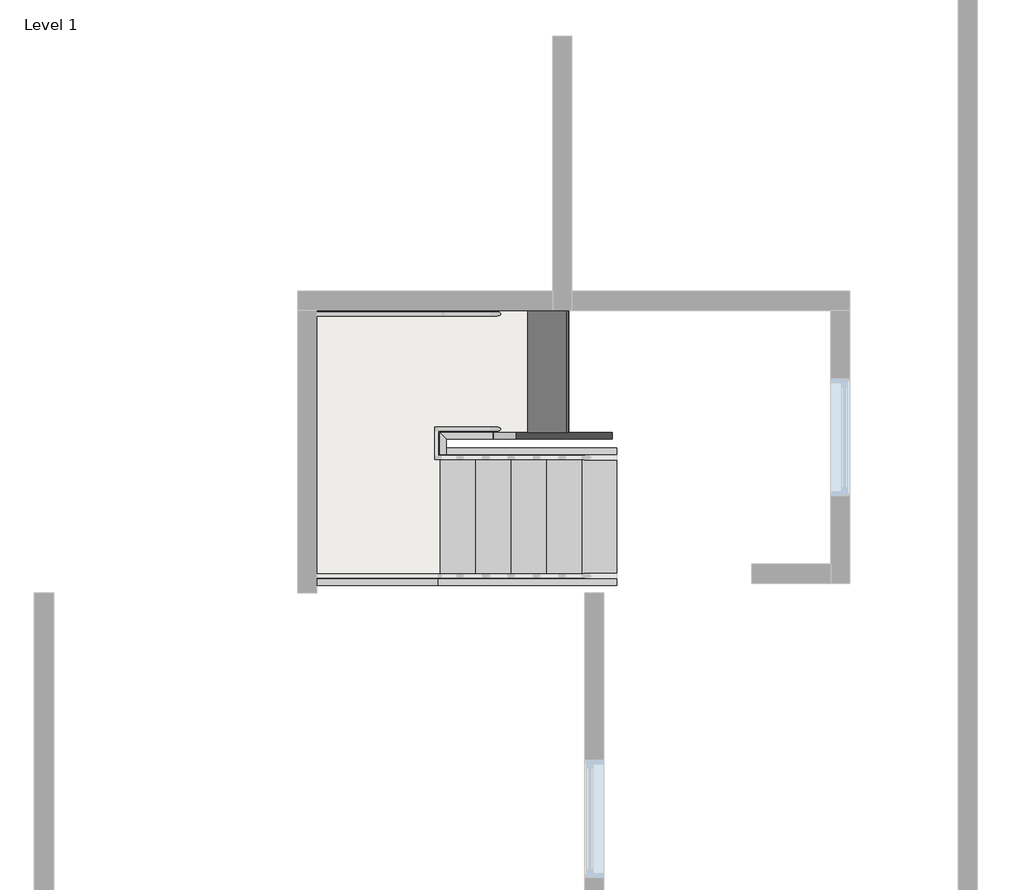
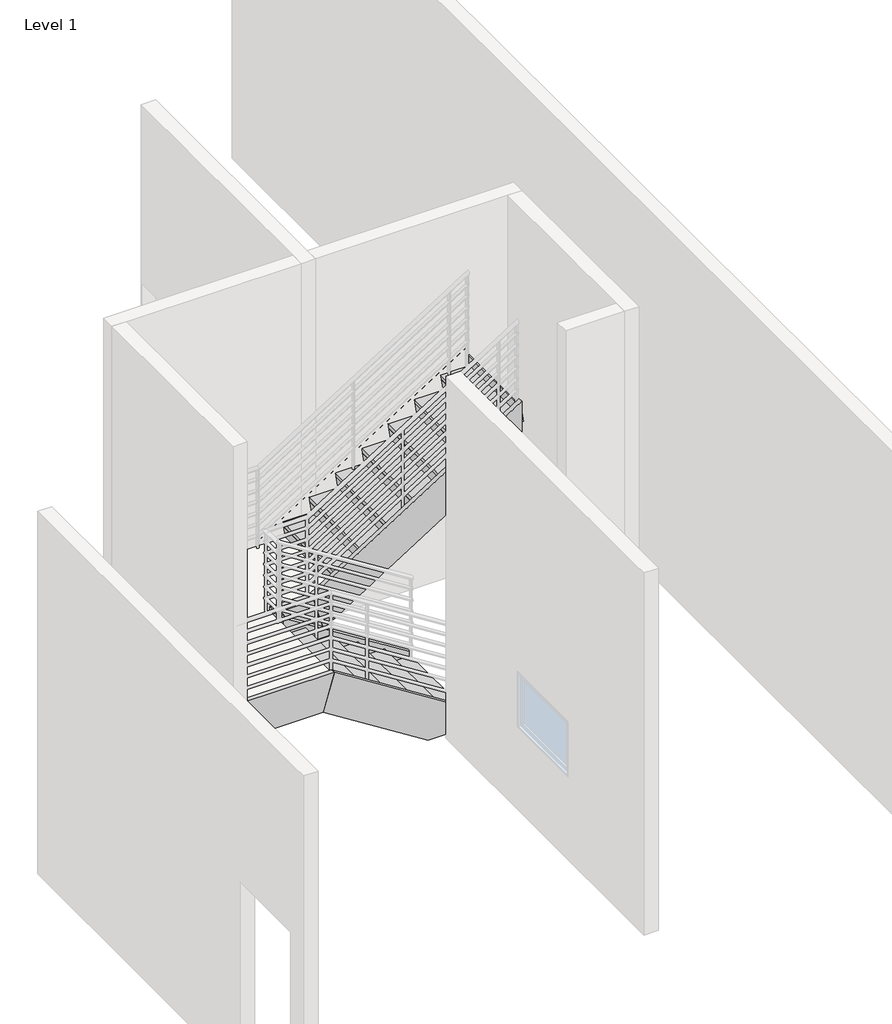
# One storey, part 4 of 4: 9 members, 2 stair flights, 1 slab.
"""IFC4 building model written with IfcOpenShell, lengths in millimetres."""

from ifc_helpers import new_model, si_unit, frame, origin, place, context, project, spatial, polyline, outline, extrude, faceted_brep, transform, mapped, element, save
from components import non_monolithic_landing_e0a5ec0f, stair_flight_50mm_tread_25mm_nosing_13mm_riser_d346f2b6, stair_flight_50mm_tread_25mm_nosing_13mm_riser_6fe2c66d

model = new_model("IFC4")

# Units and contexts
model_context = context("Model", 3, world=origin())
ifc_project = project(units=[si_unit("LENGTHUNIT", "METRE", prefix="MILLI")], contexts=[model_context])

# Site, building, storey
site = spatial("IfcSite", under=ifc_project)
building = spatial("IfcBuilding", under=site)
storey = spatial("IfcBuildingStorey", under=building, Name="Level 1", Elevation=0.0)

# Members
placement = place(None, origin())
element("IfcMember", 1, ObjectType="Stringer - 50mm Width", at=placement, inside=storey, context=model_context, shape_type="SweptSolid", body=[
    extrude(outline(polyline([(0.0, -539.0915237), (215.089535, -539.0915237), (1090.8719878, -1923.9225273), (690.8719878, -2039.7915873), (0.0, -947.3502566), (0.0, -539.0915237)])), frame((0.0, 793.0180557, 0.0), z_axis=(0.0, 1.0, 0.0), x_axis=(0.0, 0.0, 1.0)), (0.0, 0.0, 1.0), 50.0),
])
element("IfcMember", 2, ObjectType="Stringer - 50mm Width", at=placement, inside=storey, context=model_context, shape_type="SweptSolid", body=[
    extrude(outline(polyline([(0.0, -539.0915237), (215.089535, -539.0915237), (1053.034199, -1864.0915237), (579.7573231, -1864.0915237), (0.0, -947.3502566), (0.0, -539.0915237)])), frame((0.0, 1810.8567276, 0.0), z_axis=(0.0, 1.0, 0.0), x_axis=(0.0, 0.0, 1.0)), (0.0, 0.0, 1.0), 50.0),
])
element("IfcMember", 3, ObjectType="Stringer - 50mm Width", at=placement, inside=storey, context=model_context, shape_type="SweptSolid", body=[
    extrude(outline(polyline([(1090.8719878, -1497.6387118), (690.8719878, -1381.7696518), (2002.6822243, 692.5302847), (2475.9591002, 692.5302847), (1090.8719878, -1497.6387118)])), frame((0.0, 2926.2309464, 0.0), z_axis=(0.0, 1.0, 0.0), x_axis=(0.0, 0.0, 1.0)), (0.0, 0.0, 1.0), 50.0),
])
element("IfcMember", 4, ObjectType="Stringer - 50mm Width", at=placement, inside=storey, context=model_context, shape_type="SweptSolid", body=[
    extrude(outline(polyline([(1090.8719878, -1497.6387118), (690.8719878, -1381.7696518), (2002.6822243, 692.5302847), (2475.9591002, 692.5302847), (1090.8719878, -1497.6387118)])), frame((0.0, 1930.9593033, 0.0), z_axis=(0.0, 1.0, 0.0), x_axis=(0.0, 0.0, 1.0)), (0.0, 0.0, 1.0), 50.0),
])
element("IfcMember", 5, ObjectType="Stringer - 50mm Width", at=placement, inside=storey, context=model_context, shape_type="Brep", body=[
    faceted_brep([(-1497.6387118, 2926.2309464, 1090.8719878), (-1497.6387118, 2976.2309464, 1090.8719878), (-2964.117305, 2976.2309464, 1090.8719878), (-2914.117305, 2926.2309464, 1090.8719878), (-1381.7696518, 2926.2309464, 690.8719878), (-2914.117305, 2926.2309464, 690.8719878), (-1381.7696518, 2976.2309464, 690.8719878), (-2964.117305, 2976.2309464, 690.8719878)], [[[0, 1, 2, 3]], [[4, 0, 3, 5]], [[6, 4, 5, 7]], [[1, 6, 7, 2]], [[1, 0, 4, 6]], [[2, 7, 5, 3]]]),
])
element("IfcMember", 6, ObjectType="Stringer - 50mm Width", at=placement, inside=storey, context=model_context, shape_type="SweptSolid", body=[
    extrude(outline(polyline([(-2964.117305, 2976.2309464), (-2914.117305, 2926.2309464), (-2914.117305, 843.0180557), (-2964.117305, 793.0180557), (-2964.117305, 2976.2309464)])), frame((0.0, 0.0, 690.8719878), z_axis=(0.0, 0.0, 1.0), x_axis=(1.0, 0.0, 0.0)), (0.0, 0.0, 1.0), 400.0),
])
element("IfcMember", 7, ObjectType="Stringer - 50mm Width", at=placement, inside=storey, context=model_context, shape_type="Brep", body=[
    faceted_brep([(-2914.117305, 843.0180557, 1090.8719878), (-2964.117305, 793.0180557, 1090.8719878), (-1923.9225273, 793.0180557, 1090.8719878), (-1923.9225273, 843.0180557, 1090.8719878), (-2914.117305, 843.0180557, 690.8719878), (-2039.7915873, 843.0180557, 690.8719878), (-2964.117305, 793.0180557, 690.8719878), (-2039.7915873, 793.0180557, 690.8719878)], [[[0, 1, 2, 3]], [[4, 0, 3, 5]], [[6, 4, 5, 7]], [[1, 6, 7, 2]], [[1, 0, 4, 6]], [[2, 7, 5, 3]]]),
])
element("IfcMember", 8, ObjectType="Stringer - 50mm Width", at=placement, inside=storey, context=model_context, shape_type="SweptSolid", body=[
    extrude(outline(polyline([(-1864.0915237, 1810.8567276), (-1914.0915237, 1810.8567276), (-1914.0915237, 1980.9593033), (-1864.0915237, 1930.9593033), (-1864.0915237, 1810.8567276)])), frame((0.0, 0.0, 690.8719878), z_axis=(0.0, 0.0, 1.0), x_axis=(1.0, 0.0, 0.0)), (0.0, 0.0, 1.0), 400.0),
])
element("IfcMember", 9, ObjectType="Stringer - 50mm Width", at=placement, inside=storey, context=model_context, shape_type="Brep", body=[
    faceted_brep([(-1914.0915237, 1980.9593033, 1090.8719878), (-1864.0915237, 1930.9593033, 1090.8719878), (-1497.6387118, 1930.9593033, 1090.8719878), (-1497.6387118, 1980.9593033, 1090.8719878), (-1914.0915237, 1980.9593033, 690.8719878), (-1381.7696518, 1980.9593033, 690.8719878), (-1864.0915237, 1930.9593033, 690.8719878), (-1381.7696518, 1930.9593033, 690.8719878)], [[[0, 1, 2, 3]], [[4, 0, 3, 5]], [[6, 4, 5, 7]], [[1, 6, 7, 2]], [[1, 0, 4, 6]], [[2, 7, 5, 3]]]),
])

# Slab
non_monolithic_landing_shape = non_monolithic_landing_e0a5ec0f(model_context)
element("IfcSlab", 10, ObjectType="Non-Monolithic Landing", at=placement, inside=storey, context=model_context, shape_type="MappedRepresentation", body=[
    mapped(non_monolithic_landing_shape, transform((0.0, 0.0, 0.0), x_axis=(1.0, 0.0, 0.0), y_axis=(0.0, 1.0, 0.0), z_axis=(0.0, 0.0, 1.0))),
])

# Stair flights
stair_flight_50mm_tread_25mm_nosing_13mm_riser_shape = stair_flight_50mm_tread_25mm_nosing_13mm_riser_d346f2b6(model_context)
element("IfcStairFlight", 11, ObjectType="50mm Tread 25mm Nosing 13mm Riser", at=placement, inside=storey, context=model_context, shape_type="MappedRepresentation", body=[
    mapped(stair_flight_50mm_tread_25mm_nosing_13mm_riser_shape, transform((0.0, 0.0, 0.0), x_axis=(1.0, 0.0, 0.0), y_axis=(0.0, 1.0, 0.0), z_axis=(0.0, 0.0, 1.0))),
])
stair_flight_50mm_tread_25mm_nosing_13mm_riser_2_shape = stair_flight_50mm_tread_25mm_nosing_13mm_riser_6fe2c66d(model_context)
element("IfcStairFlight", 12, ObjectType="50mm Tread 25mm Nosing 13mm Riser", at=placement, inside=storey, context=model_context, shape_type="MappedRepresentation", body=[
    mapped(stair_flight_50mm_tread_25mm_nosing_13mm_riser_2_shape, transform((0.0, 0.0, 0.0), x_axis=(1.0, 0.0, 0.0), y_axis=(0.0, 1.0, 0.0), z_axis=(0.0, 0.0, 1.0))),
])

save(model, "model.ifc")

# Revit data of these elements
# Elements 1, 2, 3, 4, 5, 6, 7, 8, 9 (IfcMember, "Stringer - 50mm Width")
#   Phase Created = New Construction
# Element 10 (IfcSlab, "Non-Monolithic Landing")
#   Phase Created = New Construction
# Elements 11, 12 (IfcStairFlight, "50mm Tread 25mm Nosing 13mm Riser")
#   Phase Created = New Construction
